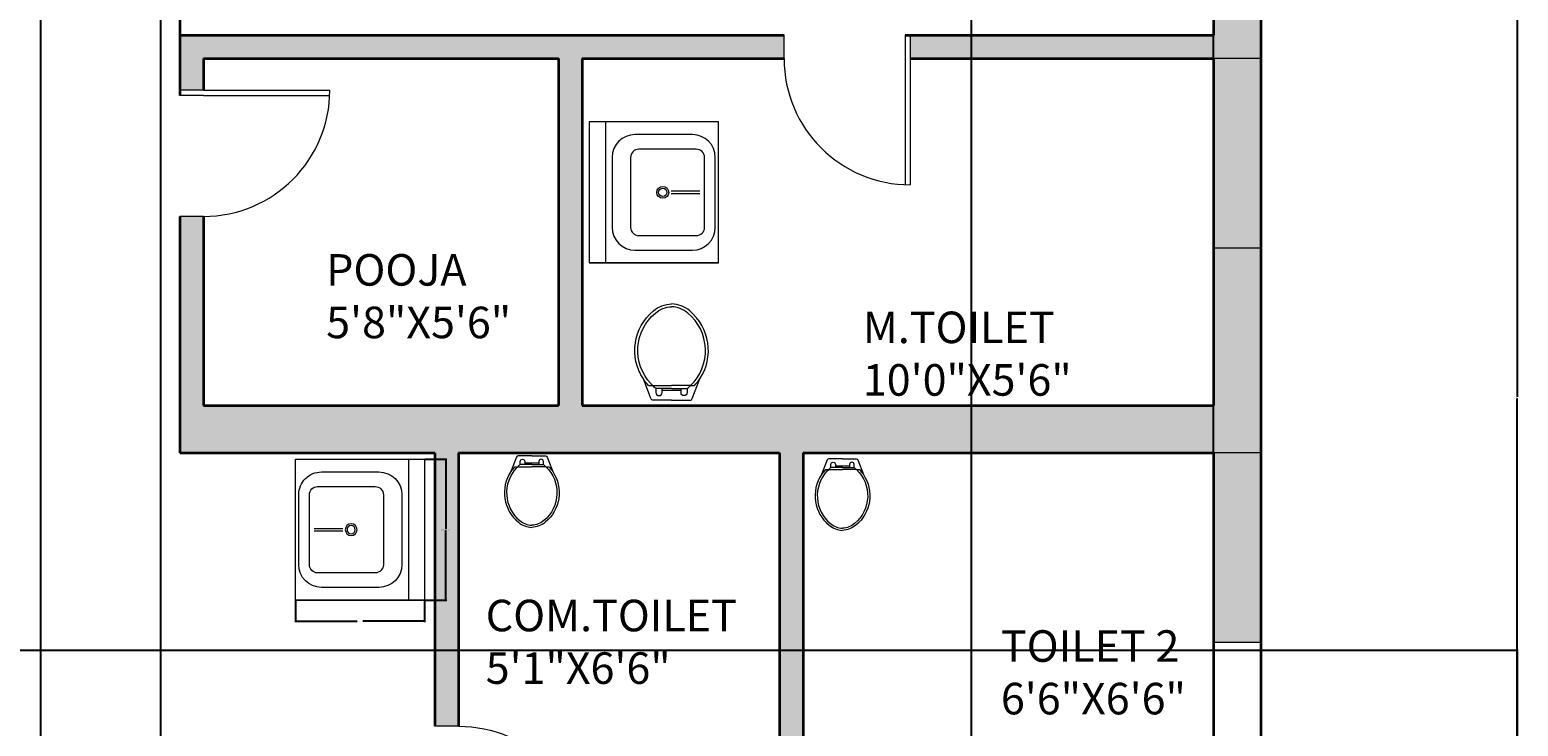
# Model space of a CAD drawing. Units: inches. Extents: x -26 to 13070, y -956 to 6917.
# Tile 10 of 13: x 314 to 597, y -286 to -154. Entities that reach past the tile are written whole.
import ezdxf

# ---------------------------------------------------------------- set-up
doc = ezdxf.new("R2010")
doc.units = ezdxf.units.IN
doc.header["$MEASUREMENT"] = 0
for name, color, linetype, lineweight in [('A-ANNO-DIMS', 2, 'Continuous', 18), ('A-AREA-IDEN', 7, 'Continuous', 18), ('A-DOOR', 3, 'Continuous', 18), ('A-FLOR-FIXT', 9, 'Continuous', 18), ('A-GLAZ', 4, 'Continuous', 18), ('A-GLAZ-PATT', 8, 'Continuous', 13), ('A-WALL', 7, 'Continuous', 35), ('A-WALL-PATT', 252, 'Continuous', 13)]:
    doc.layers.add(name, color=color, linetype=linetype, lineweight=lineweight)
doc.styles.get("Standard").update_dxf_attribs({"font": 'arial.ttf'})
doc.dimstyles.get("Standard").update_dxf_attribs({"dimtxt": 0.18, "dimasz": 0.18, "dimexe": 0.18, "dimexo": 0.0625, "dimgap": 0.09, "dimtad": 0, "dimtih": 1, "dimtoh": 1, "dimdec": 0, "dimzin": 0, "dimdsep": 46, "dimlunit": 3, "dimtxsty": 'Standard', "dimcen": 0.09, "dimadec": 0, "dimazin": 0, "dimtfac": 1, "dimtdec": 0, "dimtofl": 0, "dimtmove": 0, "dimatfit": 3, "dimfxl": 1, "dimtolj": 1, "dimtzin": 0, "dimarcsym": 0})

# ---------------------------------------------------------------- blocks, each defined once
blk = doc.blocks.new('М14 600х655')
for p, q in [((-655, 600), (-655, 0)), ((-655, 600), (-655, 0)), ((-655, 0), (-655, 600)), ((0, 600), (-655, 600)), ((0, 0), (0, 600)), ((0, 525), (-655, 525)), ((-165.1, 494.1), (-489.9, 494.1)), ((-595.8, 388.1), (-595.8, 121.3)), ((-528.4, 370.1), (-528.4, 103.3)), ((-165.4, 408.4), (-490.2, 408.4)), ((-127.2, 103.3), (-127.2, 370.1)), ((-59.2, 121.3), (-59.2, 388.1)), ((-333.5, 87.1), (-333.5, 219.6)), ((-321.5, 87.1), (-321.5, 219.6)), ((-655, 0), (-655, 0)), ((-655, 0), (-655, 0)), ((-655, 0), (0, 0)), ((-655, 0), (0, 0)), ((-490.2, 65.1), (-165.4, 65.1)), ((-489.9, 15.4), (-165.1, 15.4))]:
    blk.add_line(p, q)
for radius in [27.6, 19.3]:
    blk.add_circle((-327.5, 258.9), radius)
for centre, radius, start, end in [((-489.9, 388.1), 105.9, 90, 180), ((-165.1, 388.1), 105.9, 0, 90), ((-490.2, 370.1), 38.2, 90, 180), ((-165.4, 370.1), 38.2, 0, 90), ((-489.9, 121.3), 105.9, 180, 270), ((-490.2, 103.3), 38.2, 180, 270), ((-165.4, 103.3), 38.2, 270, 0), ((-165.1, 121.3), 105.9, 270, 0)]:
    blk.add_arc(centre, radius, start, end)
blk = doc.blocks.new('WC-COMPACT')
for p, q in [((1.95, 11.55), (2.52, 11.55)), ((2.52, 11.55), (5.2, 11.55)), ((7.87, 11.55), (5.2, 11.55)), ((7.87, 11.55), (8.44, 11.55))]:
    blk.add_line(p, q)
for points in [[(5.2, 13.61), (2.6, 13.61, 0.31031), (2.28, 13.39), (1.21, 10.61, 0.209071)], [(1.95, 11.55, 0.040937), (1.21, 10.61, 0.163732)], [(2.52, 11.55, 0.014165), (2.25, 11.27, 0.162618)], [(2.99, 11.96, 0.022712), (2.52, 11.55, 0.162618)], [(2.99, 11.96), (2.99, 12.53, -1), (3.86, 12.53), (3.86, 12.23)], [(5.2, 11.96), (2.99, 11.96, 0.022712)], [(5.2, 13.61), (7.79, 13.61, -0.31031), (8.11, 13.39), (9.18, 10.61, -0.209071)], [(5.2, 11.96), (7.4, 11.96, -0.476108)], [(7.87, 11.55, -0.448546), (7.5, 1.29, -0.162618), (5.2, 0.41, -0.470877)], [(7.4, 11.96), (7.4, 12.53, 1), (6.54, 12.53), (6.54, 12.23)], [(7.4, 11.96, -0.022712), (7.87, 11.55, -0.162618)], [(8.44, 11.55, -0.040937), (9.18, 10.61, -0.163732)], [(1.21, 10.61, 0.383919), (2.64, 0.98, 0.163732), (5.2, 0, 0.359733)], [(2.25, 11.27, 0.431639), (2.9, 1.29, 0.162618), (5.2, 0.41, 0.470877)], [(9.18, 10.61, -0.383919), (7.75, 0.98, -0.163732), (5.2, 0, -0.359733)]]:
    blk.add_lwpolyline(points, format="xyb")
for points in [[(6.54, 12.23), (3.86, 12.23)], [(3.86, 12.23), (3.86, 11.96)], [(6.54, 12.23), (6.54, 11.96)]]:
    blk.add_lwpolyline(points)
blk = doc.blocks.new('WC-STANDARD')
for p, q in [((2.62, 2.77), (3.39, 2.77)), ((3.39, 2.77), (6.99, 2.77)), ((10.59, 2.77), (6.99, 2.77)), ((10.59, 2.77), (11.36, 2.77))]:
    blk.add_line(p, q)
for points in [[(1.63, 4.03, -0.383919), (3.55, 16.99, -0.163732), (6.99, 18.31, -0.359733)], [(3.02, 3.15, -0.431639), (3.9, 16.57, -0.162618), (6.99, 17.76, -0.470877)], [(12.35, 4.03, 0.383919), (10.43, 16.99, 0.163732), (6.99, 18.31, 0.359733)], [(10.59, 2.77, 0.448546), (10.08, 16.57, 0.162618), (6.99, 17.76, 0.470877)], [(2.62, 2.77, -0.040937), (1.63, 4.03, -0.163732)], [(6.99, 0), (3.49, 0, -0.31031), (3.07, 0.29), (1.63, 4.03, -0.209071)], [(3.39, 2.77, -0.014165), (3.02, 3.15, -0.162618)], [(6.99, 0), (10.49, 0, 0.31031), (10.92, 0.29), (12.35, 4.03, 0.209071)], [(11.36, 2.77, 0.040937), (12.35, 4.03, 0.163732)], [(4.02, 2.22, -0.022712), (3.39, 2.77, -0.162618)], [(6.99, 2.22), (4.02, 2.22, -0.022712)], [(4.02, 2.22), (4.02, 1.45, 1), (5.19, 1.45), (5.19, 1.85)], [(6.99, 2.22), (9.96, 2.22, 0.476108)], [(9.96, 2.22), (9.96, 1.45, -1), (8.79, 1.45), (8.79, 1.85)], [(9.96, 2.22, 0.022712), (10.59, 2.77, 0.162618)]]:
    blk.add_lwpolyline(points, format="xyb")
for points in [[(5.19, 1.85), (5.19, 2.22)], [(8.79, 1.85), (5.19, 1.85)], [(8.79, 1.85), (8.79, 2.22)]]:
    blk.add_lwpolyline(points)
blk = doc.blocks.new('DOOR-SWING-24')
for p, q in [((24, 1), (0, 1)), ((24, 0), (0, 0))]:
    blk.add_line(p, q)
blk.add_arc((24, 0), 24, 90, 180)
blk = doc.blocks.new('*D24')
at = {"layer": 'A-ANNO-DIMS', "color": 0, "lineweight": -2, "transparency": 16777216}
for p, q in [((388.74, -235.23), (392.88, -235.23)), ((392.7, -235.41), (392.7, -248.46)), ((392.7, -261.88), (392.7, -248.83)), ((388.74, -262.06), (392.88, -262.06))]:
    blk.add_line(p, q, dxfattribs=at)
at = {"layer": 'A-ANNO-DIMS', "color": 0, "transparency": 16777216}
for points in [[(392.67, -235.41), (392.73, -235.41), (392.7, -235.23)], [(392.67, -261.88), (392.73, -261.88), (392.7, -262.06)]]:
    blk.add_solid(points, dxfattribs=at)
at = {"layer": 'Defpoints', "color": 0, "transparency": 16777216}
for p in [(388.67, -235.23), (392.7, -235.23), (388.67, -262.06)]:
    blk.add_point(p, dxfattribs=at)
at = {"layer": 'A-ANNO-DIMS', "color": 0, "transparency": 16777216, "insert": (392.7, -248.65), "char_height": 0.18, "attachment_point": 5}
blk.add_mtext('\\A1;BASIN 27 TYP.', dxfattribs=at)
blk = doc.blocks.new('*D25')
at = {"layer": 'A-ANNO-DIMS', "color": 0, "lineweight": -2, "transparency": 16777216}
for p, q in [((364.1, -262.12), (364.1, -266.26)), ((388.67, -262.12), (388.67, -266.26)), ((364.28, -266.08), (375.86, -266.08)), ((388.49, -266.08), (376.92, -266.08))]:
    blk.add_line(p, q, dxfattribs=at)
at = {"layer": 'A-ANNO-DIMS', "color": 0, "transparency": 16777216}
for points in [[(364.28, -266.05), (364.28, -266.11), (364.1, -266.08)], [(388.49, -266.05), (388.49, -266.11), (388.67, -266.08)]]:
    blk.add_solid(points, dxfattribs=at)
at = {"layer": 'Defpoints', "color": 0, "transparency": 16777216}
for p in [(364.1, -262.06), (388.67, -262.06), (388.67, -266.08)]:
    blk.add_point(p, dxfattribs=at)
at = {"layer": 'A-ANNO-DIMS', "color": 0, "transparency": 16777216, "insert": (376.39, -266.08), "char_height": 0.18, "attachment_point": 5}
blk.add_mtext('\\A1;25 TYP.', dxfattribs=at)
blk = doc.blocks.new('*D45')
at = {"layer": 'A-ANNO-DIMS', "color": 0, "lineweight": -2, "transparency": 16777216}
for p, q in [((547.7, 10.46), (596.57, 10.46)), ((596.39, 10.28), (596.39, -223.36)), ((596.39, -457.36), (596.39, -223.72)), ((538.7, -457.54), (596.57, -457.54))]:
    blk.add_line(p, q, dxfattribs=at)
at = {"layer": 'A-ANNO-DIMS', "color": 0, "transparency": 16777216}
for points in [[(596.36, 10.28), (596.42, 10.28), (596.39, 10.46)], [(596.36, -457.36), (596.42, -457.36), (596.39, -457.54)]]:
    blk.add_solid(points, dxfattribs=at)
at = {"layer": 'Defpoints', "color": 0, "transparency": 16777216}
for p in [(547.64, 10.46), (596.39, 10.46), (538.64, -457.54)]:
    blk.add_point(p, dxfattribs=at)
at = {"layer": 'A-ANNO-DIMS', "color": 0, "transparency": 16777216, "insert": (596.39, -223.54), "char_height": 0.18, "attachment_point": 5}
blk.add_mtext('\\A1;468', dxfattribs=at)
blk = doc.blocks.new('*D50')
at = {"layer": 'A-ANNO-DIMS', "color": 0, "lineweight": -2, "transparency": 16777216}
for p, q in [((315.7, -495.61), (315.7, 116.39)), ((315.88, 116.21), (326.72, 116.21)), ((338.35, 116.21), (327.51, 116.21)), ((338.53, -495.61), (338.53, 116.39))]:
    blk.add_line(p, q, dxfattribs=at)
at = {"layer": 'A-ANNO-DIMS', "color": 0, "transparency": 16777216}
for points in [[(315.88, 116.24), (315.88, 116.18), (315.7, 116.21)], [(338.35, 116.24), (338.35, 116.18), (338.53, 116.21)]]:
    blk.add_solid(points, dxfattribs=at)
at = {"layer": 'Defpoints', "color": 0, "transparency": 16777216}
for p in [(338.53, 116.21), (315.7, -495.67), (338.53, -495.67)]:
    blk.add_point(p, dxfattribs=at)
at = {"layer": 'A-ANNO-DIMS', "color": 0, "transparency": 16777216, "insert": (327.12, 116.21), "char_height": 0.18, "attachment_point": 5}
blk.add_mtext('\\A1;22.83', dxfattribs=at)
blk = doc.blocks.new('*D53')
at = {"layer": 'A-ANNO-DIMS', "color": 0, "lineweight": -2, "transparency": 16777216}
for p, q in [((492.64, -622.48), (492.64, 116.39)), ((492.82, 116.21), (515.42, 116.21)), ((538.46, 116.21), (515.86, 116.21)), ((538.64, -622.48), (538.64, 116.39))]:
    blk.add_line(p, q, dxfattribs=at)
at = {"layer": 'A-ANNO-DIMS', "color": 0, "transparency": 16777216}
for points in [[(492.82, 116.24), (492.82, 116.18), (492.64, 116.21)], [(538.46, 116.24), (538.46, 116.18), (538.64, 116.21)]]:
    blk.add_solid(points, dxfattribs=at)
at = {"layer": 'Defpoints', "color": 0, "transparency": 16777216}
for p in [(538.64, 116.21), (492.64, -622.54), (538.64, -622.54)]:
    blk.add_point(p, dxfattribs=at)
at = {"layer": 'A-ANNO-DIMS', "color": 0, "transparency": 16777216, "insert": (515.64, 116.21), "char_height": 0.18, "attachment_point": 5}
blk.add_mtext('\\A1;46', dxfattribs=at)
blk = doc.blocks.new('*D57')
at = {"layer": 'A-ANNO-DIMS', "color": 0, "lineweight": -2, "transparency": 16777216}
for p, q in [((154.7, -271.54), (596.57, -271.54)), ((596.39, -271.72), (596.39, -351.36)), ((596.39, -431.36), (596.39, -351.72)), ((154.7, -431.54), (596.57, -431.54))]:
    blk.add_line(p, q, dxfattribs=at)
at = {"layer": 'A-ANNO-DIMS', "color": 0, "transparency": 16777216}
for points in [[(596.36, -271.72), (596.42, -271.72), (596.39, -271.54)], [(596.36, -431.36), (596.42, -431.36), (596.39, -431.54)]]:
    blk.add_solid(points, dxfattribs=at)
at = {"layer": 'Defpoints', "color": 0, "transparency": 16777216}
for p in [(154.64, -271.54), (596.39, -271.54), (154.64, -431.54)]:
    blk.add_point(p, dxfattribs=at)
at = {"layer": 'A-ANNO-DIMS', "color": 0, "transparency": 16777216, "insert": (596.39, -351.54), "char_height": 0.18, "attachment_point": 5}
blk.add_mtext('\\A1;160', dxfattribs=at)

msp = doc.modelspace()

# ---------------------------------------------------------------- hatches: boundary and pattern name
at = {"layer": 'A-GLAZ-PATT'}
h = msp.add_hatch(dxfattribs=at)
h.set_pattern_fill('GOST_WOOD', color=256)
h.set_pattern_definition([(90, (0, 0), (6, -4e-16), [10, -2]), (90, (2, -2), (6, -4e-16), [6, -1.5, 3, -1.5]), (90, (4, -5), (6, -4e-16), [10, -2])])
h.paths.add_polyline_path([(547.641, -159.042), (538.641, -159.042), (538.641, -195.042), (547.641, -195.042)])
h.paths.add_polyline_path([(547.641, -234.042), (538.641, -234.042), (538.641, -270.042), (547.641, -270.042)])
h.paths.add_polyline_path([(547.641, -654.042), (538.641, -654.042), (538.641, -690.042), (547.641, -690.042)])
at = {"layer": 'A-WALL-PATT'}
h = msp.add_hatch(color=256, dxfattribs=at)
h.dxf.hatch_style = 1
h.paths.add_polyline_path([(223.641, 10.458), (214.641, 10.458), (22.641, 10.458), (22.641, -171.042), (31.641, -171.042), (31.641, -135.042), (205.641, -135.042), (205.641, -241.042), (210.141, -241.042), (210.141, -130.542), (94.641, -130.542), (94.641, -76.542), (85.641, -76.542), (85.641, -126.042), (27.141, -126.042), (27.141, 5.958), (85.641, 5.958), (85.641, -52.542), (94.641, -52.542), (94.641, 1.458), (214.641, 1.458), (214.641, -16.542), (223.641, -16.542), (229.641, -16.542), (229.641, -7.542), (223.641, -7.542)])
h.paths.add_polyline_path([(367.048, 10.458), (346.641, 10.458), (337.641, 10.458), (337.641, -7.542), (331.641, -7.542), (331.641, -16.542), (337.641, -16.542), (342.141, -16.542), (342.141, -128.542), (346.641, -128.542), (346.641, 1.458), (367.048, 1.458)])
h.paths.add_polyline_path([(547.641, 10.458), (403.048, 10.458), (403.048, 1.458), (538.641, 1.458), (538.641, -46.542), (547.641, -46.542)])
h.paths.add_polyline_path([(547.641, -106.542), (538.641, -106.542), (538.641, -154.542), (481.013, -154.542), (481.013, -159.042), (538.641, -159.042), (547.641, -159.042)])
h.paths.add_polyline_path([(457.013, -154.542), (342.141, -154.542), (342.141, -165.042), (346.641, -165.042), (346.641, -159.042), (414.141, -159.042), (414.141, -225.042), (346.641, -225.042), (346.641, -189.042), (342.141, -189.042), (342.141, -234.042), (390.641, -234.042), (390.641, -286.042), (395.141, -286.042), (395.141, -234.042), (456.141, -234.042), (456.141, -312.042), (372.641, -312.042), (372.641, -316.542), (462.641, -316.542), (462.641, -312.042), (460.641, -312.042), (460.641, -234.042), (538.641, -234.042), (547.641, -234.042), (547.641, -195.042), (538.641, -195.042), (538.641, -225.042), (418.641, -225.042), (418.641, -159.042), (457.013, -159.042)])
h.paths.add_polyline_path([(547.641, -270.042), (538.641, -270.042), (538.641, -312.042), (486.641, -312.042), (486.641, -316.542), (538.641, -316.542), (547.641, -316.542)], flags=0)
h.paths.add_polyline_path([(547.641, -456.306), (538.641, -456.306), (538.641, -457.542), (346.641, -457.542), (346.641, -316.542), (346.641, -312.042), (342.141, -312.042), (342.141, -457.542), (145.641, -457.542), (145.641, -466.542), (342.141, -466.542), (342.141, -627.042), (346.641, -627.042), (346.641, -466.542), (538.641, -466.542), (538.641, -514.542), (547.641, -514.542)])
h.paths.add_polyline_path([(466.641, -622.542), (372.641, -622.542), (372.641, -627.042), (388.641, -627.042), (388.641, -721.542), (393.141, -721.542), (393.141, -627.042), (462.141, -627.042), (462.141, -717.042), (466.641, -717.042)])
h.paths.add_polyline_path([(547.641, -574.542), (538.641, -574.542), (538.641, -622.542), (492.641, -622.542), (492.641, -627.042), (538.641, -627.042), (538.641, -654.042), (547.641, -654.042)])
h.paths.add_polyline_path([(547.641, -690.042), (538.641, -690.042), (538.641, -717.042), (466.641, -717.042), (466.641, -721.542), (538.641, -721.542), (538.641, -763.542), (547.641, -763.542)])
h.paths.add_polyline_path([(462.141, -717.042), (419.141, -717.042), (419.141, -721.542), (462.141, -721.542)], flags=0)
h.paths.add_polyline_path([(346.641, -721.542), (352.641, -721.542), (352.641, -717.042), (342.141, -717.042), (342.141, -874.542), (342.141, -907.542), (351.141, -907.542), (351.141, -874.542), (395.949, -874.542), (395.949, -865.542), (351.141, -865.542), (351.141, -841.542), (346.641, -841.542)])
h.paths.add_polyline_path([(547.641, -823.542), (538.641, -823.542), (538.641, -865.542), (431.949, -865.542), (431.949, -874.542), (547.641, -874.542)])
h.paths.add_polyline_path([(172.641, -865.713), (140.641, -865.744), (140.641, -788.744), (182.646, -788.704), (182.641, -784.204), (136.141, -784.249), (136.141, -848.332), (131.641, -848.332), (131.641, -874.542), (172.641, -874.542)])
h.paths.add_polyline_path([(217.641, -816.13), (213.141, -816.13), (213.141, -784.174), (208.641, -784.179), (208.641, -865.679), (208.641, -874.542), (217.641, -874.542)])
h.paths.add_polyline_path([(95.641, -865.788), (31.641, -865.849), (31.641, -832.695), (22.641, -832.695), (22.641, -874.542), (95.641, -874.542)])
h.paths.add_polyline_path([(217.641, -741.17), (31.641, -741.349), (31.641, -708.349), (22.641, -708.349), (22.641, -772.542), (22.641, -796.695), (31.641, -796.695), (31.641, -763.542), (31.641, -745.849), (217.641, -745.67)])
h.paths.add_polyline_path([(31.641, -651.349), (99.65, -651.284), (99.641, -642.284), (31.641, -642.349), (31.641, -639.042), (31.641, -588.349), (125.641, -588.259), (125.641, -651.259), (134.641, -651.25), (134.641, -579.25), (112.641, -579.271), (112.641, -549.042), (112.641, -504.271), (85.633, -504.297), (85.641, -513.297), (103.641, -513.28), (103.641, -549.042), (103.641, -579.28), (31.641, -579.349), (31.641, -549.042), (31.641, -513.349), (49.641, -513.314), (49.633, -504.332), (31.641, -504.349), (22.641, -504.358), (22.641, -684.349), (31.641, -684.349)])
h.paths.add_polyline_path([(31.641, -276.042), (145.641, -276.042), (145.641, -402.042), (145.641, -419.542), (154.641, -419.542), (154.641, -411.042), (154.641, -271.542), (210.141, -271.542), (210.141, -265.042), (205.641, -265.042), (205.641, -267.042), (31.641, -267.042), (31.641, -231.042), (22.641, -231.042), (22.641, -426.852), (31.641, -426.852), (31.641, -411.042), (31.641, -402.042)])

# ---------------------------------------------------------------- linework, layer by layer
at = {"layer": 'A-DOOR'}
for p, q in [((457.013, -159.042), (457.013, -154.542)), ((480.013, -154.542), (480.013, -159.042)), ((481.013, -154.542), (481.013, -159.042)), ((346.641, -165.042), (342.141, -165.042)), ((346.641, -166.042), (342.141, -166.042)), ((346.641, -189.042), (342.141, -189.042)), ((395.141, -286.042), (390.641, -286.042))]:
    msp.add_line(p, q, dxfattribs=at)
at = {"layer": 'A-GLAZ'}
for p, q in [((538.641, -159.042), (538.641, -195.042)), ((547.641, -159.042), (538.641, -159.042)), ((547.641, -195.042), (547.641, -159.042)), ((538.641, -195.042), (547.641, -195.042)), ((538.641, -234.042), (538.641, -270.042)), ((547.641, -234.042), (538.641, -234.042)), ((547.641, -270.042), (547.641, -234.042)), ((538.641, -270.042), (547.641, -270.042))]:
    msp.add_line(p, q, dxfattribs=at)
at = {"layer": 'A-WALL'}
for p, q in [((547.641, 10.458), (547.641, -874.542)), ((538.641, 1.458), (538.641, -154.542)), ((342.141, -151.542), (342.141, -166.042)), ((342.141, -154.542), (457.013, -154.542)), ((480.013, -154.542), (538.641, -154.542)), ((346.641, -159.042), (414.141, -159.042)), ((346.641, -159.042), (346.641, -165.042)), ((414.141, -159.042), (414.141, -225.042)), ((418.641, -159.042), (418.641, -225.042)), ((418.641, -159.042), (457.013, -159.042)), ((481.013, -159.042), (538.641, -159.042)), ((538.641, -159.042), (538.641, -225.042)), ((342.141, -189.042), (342.141, -234.042)), ((346.641, -189.042), (346.641, -225.042)), ((346.641, -225.042), (414.141, -225.042)), ((418.641, -225.042), (538.641, -225.042)), ((342.141, -234.042), (390.641, -234.042)), ((390.641, -234.042), (390.641, -286.042)), ((395.141, -234.042), (395.141, -286.042)), ((395.141, -234.042), (456.141, -234.042)), ((456.141, -234.042), (456.141, -312.042)), ((460.641, -234.042), (460.641, -312.042)), ((460.641, -234.042), (538.641, -234.042)), ((538.641, -234.042), (538.641, -312.042))]:
    msp.add_line(p, q, dxfattribs=at)

# ---------------------------------------------------------------- block references
at = {"layer": 'A-DOOR'}
for p, rotation in [((481.013, -183.042), 90), ((370.641, -165.041), 180)]:
    msp.add_blockref('DOOR-SWING-24', p, dxfattribs=dict(at, rotation=rotation))
at = {"layer": 'A-DOOR', "extrusion": (0, 0, -1), "zscale": -1}
msp.add_blockref('DOOR-SWING-24', (-419.141, -310.042), dxfattribs=at)
at = {"layer": 'A-FLOR-FIXT', "yscale": 0.0409591733592258, "zscale": 0.0409591733592258}
for p, xscale, rotation in [((444.559, -171.065), 0.0409591733592258, 90), ((364.098, -235.232), -0.0409591733592258, 270)]:
    msp.add_blockref('М14 600х655', p, dxfattribs=dict(at, xscale=xscale, rotation=rotation))
at = {"layer": 'A-FLOR-FIXT'}
for name, p in [('WC-STANDARD', (428.635, -224.002)), ('WC-COMPACT', (403.852, -248.211)), ('WC-COMPACT', (462.92, -248.778))]:
    msp.add_blockref(name, p, dxfattribs=at)

# ---------------------------------------------------------------- texts
at = {"layer": 'A-AREA-IDEN', "char_height": 6, "attachment_point": 1}
for s, insert in [('POOJA\\P5\'8"X5\'6"', (369.954, -196.223)), ('M.TOILET\\P10\'0"X5\'6"', (471.992, -207.16)), ('COM.TOILET\\P5\'1"X6\'6"', (400.287, -261.977)), ('TOILET 2\\P6\'6"X6\'6"', (498.241, -267.784))]:
    msp.add_mtext(s, dxfattribs=dict(at, insert=insert))

# ---------------------------------------------------------------- dimensions: what is measured, and where the dimension line sits
at = {"layer": 'A-ANNO-DIMS'}
for base, p1, p2, override, picture, middle in [((338.531, 116.209), (315.7, -495.668), (338.531, -495.668), {"dimdec": 2, "dimlfac": 1, "dimrnd": 0, "dimzin": 0, "dimdsep": 46, "dimlunit": 2}, '*D50', (327.115, 116.209)), ((538.641, 116.209), (492.641, -622.542), (538.641, -622.542), {"dimdec": 0, "dimlfac": 1, "dimrnd": 0, "dimzin": 0, "dimdsep": 46, "dimlunit": 2}, '*D53', (515.641, 116.209))]:
    dim = msp.add_linear_dim(base=base, p1=p1, p2=p2, dimstyle='Standard', override=override, dxfattribs=at)
    dim.commit()
    dim.dimension.update_dxf_attribs({"geometry": picture, "text_midpoint": middle})
for base, p1, p2, picture, middle in [((596.392, 10.458), (538.641, -457.542), (547.641, 10.458), '*D45', (596.392, -223.542)), ((596.392, -271.542), (154.641, -431.542), (154.641, -271.542), '*D57', (596.392, -351.542))]:
    dim = msp.add_linear_dim(base=base, p1=p1, p2=p2, angle=90, dimstyle='Standard', override={"dimdec": 0, "dimlfac": 1, "dimrnd": 0, "dimzin": 0, "dimdsep": 46, "dimlunit": 2}, dxfattribs=at)
    dim.commit()
    dim.dimension.update_dxf_attribs({"geometry": picture, "text_midpoint": middle})
dim = msp.add_linear_dim(base=(392.698, -235.232), p1=(388.674, -262.06), p2=(388.674, -235.232), angle=90, text='BASIN <> TYP.', dimstyle='Standard', override={"dimdec": 0, "dimlfac": 1, "dimrnd": 0, "dimzin": 0, "dimdsep": 46, "dimlunit": 2}, dxfattribs=at)
dim.commit()
dim.dimension.update_dxf_attribs({"geometry": '*D24', "text_midpoint": (392.698, -248.646)})
dim = msp.add_linear_dim(base=(388.674, -266.084), p1=(364.098, -262.06), p2=(388.674, -262.06), text='<> TYP.', dimstyle='Standard', override={"dimdec": 0, "dimlfac": 1, "dimrnd": 0, "dimzin": 0, "dimdsep": 46, "dimlunit": 2}, dxfattribs=at)
dim.commit()
dim.dimension.update_dxf_attribs({"geometry": '*D25', "text_midpoint": (376.386, -266.084)})

doc.saveas('drawing.dxf')
